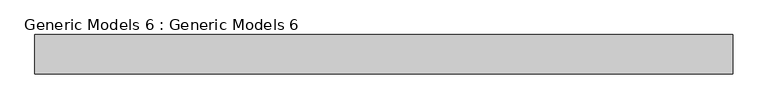
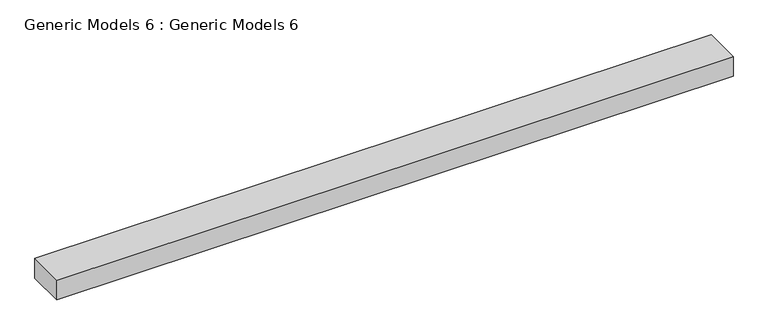
"""IFC4 building model written with IfcOpenShell, lengths in millimetres: proxy geometry, Generic Models 6 : Generic Models 6."""

from ifc_helpers import new_model, si_unit, frame, origin, place, context, project, spatial, polyline, outline, extrude, source, transform, mapped, element, save


def generic_models_6_generic_models_6_4e89bfb7(model_context):
    return source(origin(), model_context, "Body", "SweptSolid", [
        extrude(outline(polyline([(3207.6081685, -21458.2159512), (-7701.088074, -21458.2159512), (-7701.088074, -20845.7985361), (3207.6081685, -20845.7985361), (3207.6081685, -21458.2159512)])), frame((0.0, 0.0, 19474.6913921), z_axis=(0.0, 0.0, 1.0), x_axis=(1.0, 0.0, 0.0)), (0.0, 0.0, 1.0), 337.3086079),
    ])


if __name__ == "__main__":
    model = new_model("IFC4")
    model_context = context("Model", 3, world=origin())
    ifc_project = project(units=[si_unit("LENGTHUNIT", "METRE", prefix="MILLI")], contexts=[model_context])
    site = spatial("IfcSite", under=ifc_project)
    building = spatial("IfcBuilding", under=site)
    placement = place(None, origin())
    generic_models_6_generic_models_6_shape = generic_models_6_generic_models_6_4e89bfb7(model_context)
    element("IfcBuildingElementProxy", 1, Name="Generic Models 6 : Generic Models 6", ObjectType="Generic Models 6 : Generic Models 6", at=placement, inside=building, context=model_context, shape_type="MappedRepresentation", body=[
        mapped(generic_models_6_generic_models_6_shape, transform((0.0, 0.0, 0.0), x_axis=(1.0, 0.0, 0.0), y_axis=(0.0, 1.0, 0.0), z_axis=(0.0, 0.0, 1.0))),
    ])
    save(model, "model.ifc")
